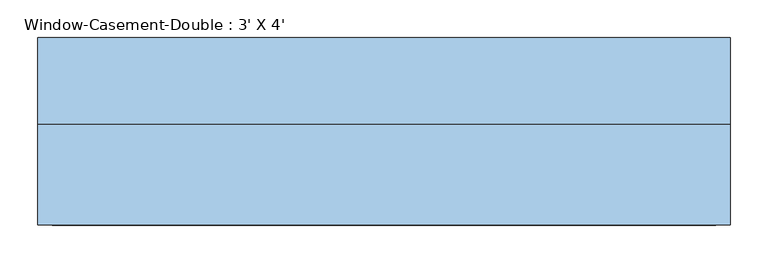
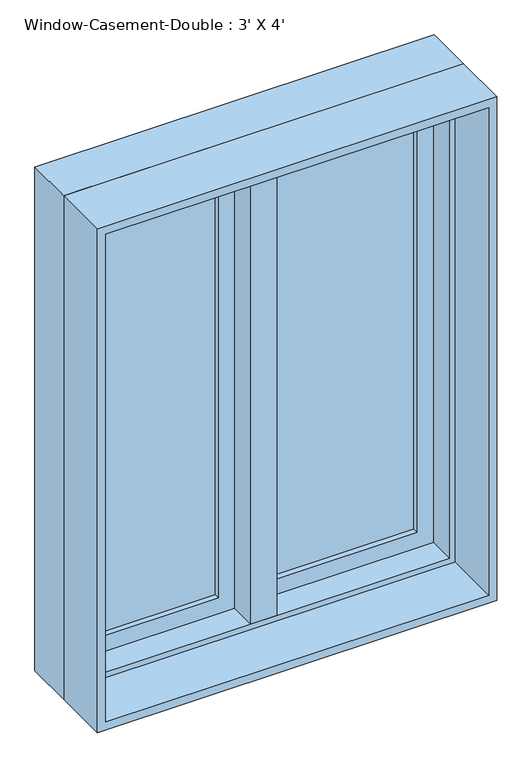
"""IFC4 building model written with IfcOpenShell, lengths in millimetres: window geometry, Window-Casement-Double : 3' X 4'."""

from ifc_helpers import new_model, si_unit, frame, origin, place, context, project, spatial, polyline, outline, extrude, faceted_brep, source, transform, mapped, element, save


def window_casement_double_3_x_4_2abbe05e(model_context):
    return source(origin(), model_context, "Body", "SolidModel", [
        faceted_brep([(425.45, 82.55, 2101.85), (425.45, 19.05, 2101.85), (-425.45, 19.05, 2101.85), (-425.45, 82.55, 2101.85), (444.5, 133.35, 2120.9), (444.5, 82.55, 2120.9), (-444.5, 82.55, 2120.9), (-444.5, 133.35, 2120.9), (457.2, 19.05, 2133.6), (457.2, 133.35, 2133.6), (-457.2, 133.35, 2133.6), (-457.2, 19.05, 2133.6), (-425.45, 19.05, 946.15), (-425.45, 82.55, 946.15), (-444.5, 82.55, 927.1), (-444.5, 133.35, 927.1), (-457.2, 133.35, 914.4), (-457.2, 19.05, 914.4), (425.45, 19.05, 946.15), (425.45, 82.55, 946.15), (444.5, 82.55, 927.1), (444.5, 133.35, 927.1), (457.2, 133.35, 914.4), (457.2, 19.05, 914.4)], [[[0, 1, 2, 3]], [[4, 5, 6, 7]], [[8, 9, 10, 11]], [[3, 2, 12, 13]], [[7, 6, 14, 15]], [[11, 10, 16, 17]], [[13, 12, 18, 19]], [[15, 14, 20, 21]], [[17, 16, 22, 23]], [[11, 17, 23, 8], [1, 18, 12, 2]], [[19, 18, 1, 0]], [[5, 20, 14, 6], [3, 13, 19, 0]], [[21, 20, 5, 4]], [[23, 22, 9, 8]], [[9, 22, 16, 10], [7, 15, 21, 4]]]),
        extrude(outline(polyline([(2133.6, -457.2), (914.4, -457.2), (914.4, 457.2), (2133.6, 457.2), (2133.6, -457.2)]), holes=[polyline([(2114.55, 438.15), (933.45, 438.15), (933.45, -438.15), (2114.55, -438.15), (2114.55, 438.15)])]), frame((0.0, -114.3, 0.0), z_axis=(0.0, 1.0, 0.0), x_axis=(0.0, 0.0, 1.0)), (0.0, 0.0, 1.0), 133.35),
        extrude(outline(polyline([(927.1, 444.5), (2120.9, 444.5), (2120.9, 9.525), (927.1, 9.525), (927.1, 444.5)]), holes=[polyline([(984.25, 66.675), (2063.75, 66.675), (2063.75, 387.35), (984.25, 387.35), (984.25, 66.675)])]), frame((0.0, 82.55, 0.0), z_axis=(0.0, 1.0, 0.0), x_axis=(0.0, 0.0, 1.0)), (0.0, 0.0, 1.0), 44.45),
        extrude(outline(polyline([(2120.9, -444.5), (927.1, -444.5), (927.1, -9.525), (2120.9, -9.525), (2120.9, -444.5)]), holes=[polyline([(2063.75, -66.675), (984.25, -66.675), (984.25, -387.35), (2063.75, -387.35), (2063.75, -66.675)])]), frame((0.0, 82.55, 0.0), z_axis=(0.0, 1.0, 0.0), x_axis=(0.0, 0.0, 1.0)), (0.0, 0.0, 1.0), 44.45),
        extrude(outline(polyline([(387.35, 114.3), (387.35, 107.95), (66.675, 107.95), (66.675, 114.3), (387.35, 114.3)])), frame((0.0, 0.0, 984.25), z_axis=(0.0, 0.0, 1.0), x_axis=(1.0, 0.0, 0.0)), (0.0, 0.0, 1.0), 1079.5),
        extrude(outline(polyline([(66.675, 95.25), (66.675, 101.6), (387.35, 101.6), (387.35, 95.25), (66.675, 95.25)])), frame((0.0, 0.0, 984.25), z_axis=(0.0, 0.0, 1.0), x_axis=(1.0, 0.0, 0.0)), (0.0, 0.0, 1.0), 1079.5),
        extrude(outline(polyline([(-66.675, 114.3), (-66.675, 107.95), (-387.35, 107.95), (-387.35, 114.3), (-66.675, 114.3)])), frame((0.0, 0.0, 984.25), z_axis=(0.0, 0.0, 1.0), x_axis=(1.0, 0.0, 0.0)), (0.0, 0.0, 1.0), 1079.5),
        extrude(outline(polyline([(-387.35, 95.25), (-387.35, 101.6), (-66.675, 101.6), (-66.675, 95.25), (-387.35, 95.25)])), frame((0.0, 0.0, 984.25), z_axis=(0.0, 0.0, 1.0), x_axis=(1.0, 0.0, 0.0)), (0.0, 0.0, 1.0), 1079.5),
        faceted_brep([(9.525, 133.35, 2120.9), (-9.525, 133.35, 2120.9), (-9.525, 82.55, 2120.9), (9.525, 82.55, 2120.9), (9.525, 133.35, 927.1), (9.525, 82.55, 927.1), (-9.525, 82.55, 927.1), (-9.525, 133.35, 927.1), (-9.525, 82.55, 946.15), (-9.525, 82.55, 2101.85), (-30.1625, 82.55, 946.15), (-30.1625, 82.55, 2101.85), (-30.1625, 19.05, 946.15), (-30.1625, 19.05, 2101.85), (30.1625, 19.05, 946.15), (30.1625, 19.05, 2101.85), (30.1625, 82.55, 946.15), (30.1625, 82.55, 2101.85), (9.525, 82.55, 946.15), (9.525, 82.55, 2101.85)], [[[0, 1, 2, 3]], [[4, 5, 6, 7]], [[1, 0, 4, 7]], [[2, 1, 7, 6, 8, 9]], [[9, 8, 10, 11]], [[11, 10, 12, 13]], [[13, 12, 14, 15]], [[15, 14, 16, 17]], [[17, 16, 18, 19]], [[0, 3, 19, 18, 5, 4]], [[18, 8, 6, 5]], [[9, 19, 3, 2]], [[8, 18, 16, 14, 12, 10]], [[19, 9, 11, 13, 15, 17]]]),
    ])


if __name__ == "__main__":
    model = new_model("IFC4")
    model_context = context("Model", 3, world=origin())
    ifc_project = project(units=[si_unit("LENGTHUNIT", "METRE", prefix="MILLI")], contexts=[model_context])
    site = spatial("IfcSite", under=ifc_project)
    building = spatial("IfcBuilding", under=site)
    placement = place(None, origin())
    window_casement_double_3_x_4_shape = window_casement_double_3_x_4_2abbe05e(model_context)
    element("IfcWindow", 1, ObjectType="Window-Casement-Double : 3' X 4'", at=placement, inside=building, context=model_context, shape_type="MappedRepresentation", body=[
        mapped(window_casement_double_3_x_4_shape, transform((0.0, 0.0, 0.0), x_axis=(1.0, 0.0, 0.0), y_axis=(0.0, 1.0, 0.0), z_axis=(0.0, 0.0, 1.0))),
    ])
    save(model, "model.ifc")

# Revit data of these elements
# Type "Window-Casement-Double : 3' X 4'"
#   Type Mark = "20"
#   Fire Rating = "0.5h"
#   Assembly Code = "B2020100"
#   Analytic Construction = "Double glazing - domestic"
#   Frame Extension [instance default] = 0' - 0 1/4"
#   Window Inset [instance default] = 0' - 0"
#   Wall Thickness [instance default] = 0' - 6"
#   Interior Wall Closure [instance default] = 0' - 2 1/4"
#   Half Width = 1' - 6"
#   Visual Light Transmittance = 0.81
#   Thermal Resistance (R) = 1.8146 (h·ft²·°F)/BTU
#   Solar Heat Gain Coefficient = 0.76
#   Rough Width = 3' - 0 1/2"
#   Rough Height = 4' - 0 1/2"
#   Height = 4' - 0"
#   Heat Transfer Coefficient (U) = 0.5511 BTU/(h·ft²·°F)
#   Exterior Wall Closure [instance default] = 0' - 1 1/4"
#   Extension Jamb [instance default] = 0' - 2 1/4"
#   Default Sill Height = 3' - 0"
#   Width = 3' - 0"
#   Muntin Visibility = yes
#   Interior Trim Visibility [instance default] = yes
#   Exterior Trim Visibility [instance default] = yes
#   Extension Jamb Visibility [instance default] = yes
#   Interior Trim Material = Wood - Stained
#   Muntin Pattern = Muntin Pattern_2x2 : Muntin Pattern_2x2
#   Interior Trim = Trim-Window-Interior-Flat : Picture Frame
#   Interior Frame Material = Wood - Stained
#   Glass Panel Material = Glass
#   Exterior Trim Material = Clad - White
#   Exterior Trim = Trim-Window-Exterior-Flat : with Sill
#   Exterior Frame Material = Clad - White
#   Wall Closure = (empty or 0)
# Element 1 (IfcWindow, "Window-Casement-Double : 3' X 4'")
#   Wall Thickness = 0' - 9"
#   Extension Jamb = 0' - 5 1/4"
#   Materials on its faces: "Wood - Stained", "Glass", "Clad - White"
# Materials
#   "Wood - Stained": class "Wood", colour RGB 224 178 126, transparency 0, Cost = 0
#   "Glass": class "Glass", colour RGB 0 128 192, transparency 0.75, Description = "Soda Lime Glass", Cost = 0
#   "Clad - White": class "Wood", colour RGB 242 242 238, transparency 0, Cost = 0
